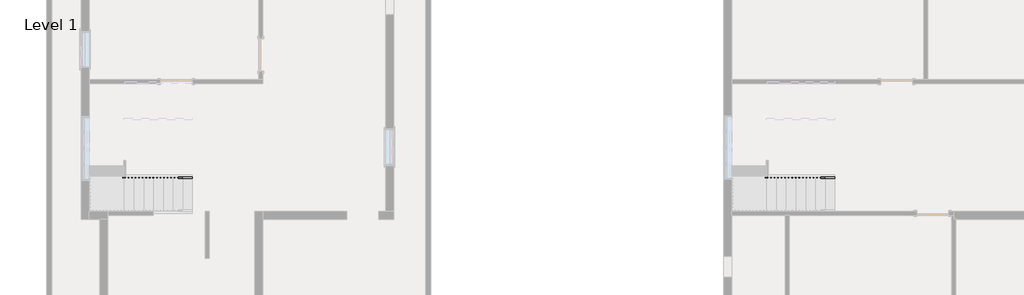
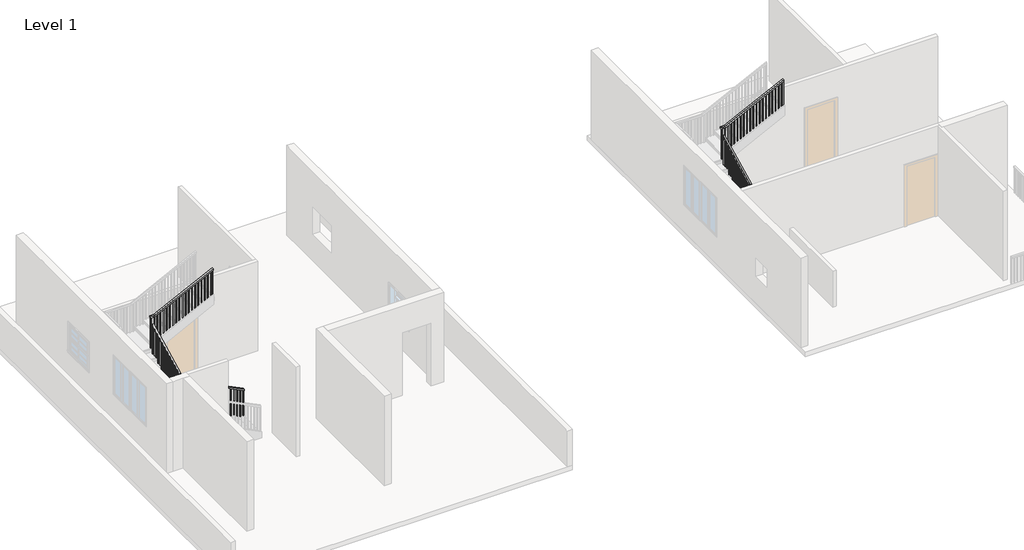
# One storey, part 4 of 8: 2 railings.
"""IFC4 building model written with IfcOpenShell, lengths in millimetres."""

from ifc_helpers import new_model, si_unit, frame, origin, place, context, project, spatial, polyline, outline, extrude, faceted_brep, element, save

model = new_model("IFC4")

# Units and contexts
model_context = context("Model", 3, world=origin())
ifc_project = project(units=[si_unit("LENGTHUNIT", "METRE", prefix="MILLI")], contexts=[model_context])

# Site, building, storey
site = spatial("IfcSite", under=ifc_project)
building = spatial("IfcBuilding", under=site)
storey = spatial("IfcBuildingStorey", under=building, Name="Level 1", Elevation=0.0)

# Railings
placement = place(None, origin())
element("IfcRailing", 1, ObjectType="Handrail - Rectangular", at=placement, inside=storey, context=model_context, shape_type="SolidModel", body=[
    faceted_brep([(-1428.1308482, -178.6399287, 1052.9454545), (-1428.1308482, -178.6399287, 996.242895), (-1428.1308482, -127.8399287, 996.242895), (-1428.1308482, -127.8399287, 1052.9454545), (-3307.7308482, -178.6399287, 1984.9785124), (-3358.5308482, -178.6399287, 1953.4660355), (-3358.5308482, -127.8399287, 1953.4660355), (-3307.7308482, -127.8399287, 1984.9785124), (-3434.7308482, -39.7364336, 2148.2942149), (-3434.7308482, -51.6399287, 2199.0942149), (-3434.7308482, 1472.3600713, 2954.7966942), (-3434.7308482, 1523.1600713, 2923.2842173), (-3383.9308482, -39.7364336, 2148.2942149), (-3383.9308482, 1523.1600713, 2923.2842173), (-3383.9308482, -51.6399287, 2199.0942149), (-3383.9308482, 1472.3600713, 2954.7966942), (-1428.1308482, 1599.3600713, 4100.9454545), (-1428.1308482, 1548.5600713, 4100.9454545), (-1428.1308482, 1548.5600713, 4044.242895), (-1428.1308482, 1599.3600713, 4044.242895), (-3295.8273531, 1599.3600713, 3118.1123967), (-3307.7308482, 1599.3600713, 3168.9123967), (-3295.8273531, 1548.5600713, 3118.1123967), (-3307.7308482, 1548.5600713, 3168.9123967), (-3307.7308482, -178.6399287, 2199.0942149), (-3358.5308482, -178.6399287, 2148.2942149), (-3358.5308482, -127.8399287, 2148.2942149), (-3307.7308482, -127.8399287, 2199.0942149), (-3434.7308482, -178.6399287, 2199.0942149), (-3434.7308482, -178.6399287, 2148.2942149), (-3383.9308482, -127.8399287, 2148.2942149), (-3383.9308482, -127.8399287, 2199.0942149), (-3434.7308482, 1472.3600713, 3168.9123967), (-3434.7308482, 1523.1600713, 3118.1123967), (-3383.9308482, 1523.1600713, 3118.1123967), (-3383.9308482, 1472.3600713, 3168.9123967), (-3434.7308482, 1599.3600713, 3168.9123967), (-3434.7308482, 1599.3600713, 3118.1123967), (-3383.9308482, 1548.5600713, 3118.1123967), (-3383.9308482, 1548.5600713, 3168.9123967)], [[[0, 1, 2, 3]], [[1, 0, 4, 5]], [[2, 1, 5, 6]], [[3, 2, 6, 7]], [[0, 3, 7, 4]], [[8, 9, 10, 11]], [[12, 8, 11, 13]], [[14, 12, 13, 15]], [[9, 14, 15, 10]], [[16, 17, 18, 19]], [[20, 21, 16, 19]], [[22, 20, 19, 18]], [[23, 22, 18, 17]], [[21, 23, 17, 16]], [[5, 4, 24, 25]], [[6, 5, 25, 26]], [[7, 6, 26, 27]], [[4, 7, 27, 24]], [[25, 24, 28, 29]], [[26, 25, 29, 30]], [[27, 26, 30, 31]], [[24, 27, 31, 28]], [[29, 28, 9, 8]], [[30, 29, 8, 12]], [[31, 30, 12, 14]], [[28, 31, 14, 9]], [[11, 10, 32, 33]], [[13, 11, 33, 34]], [[15, 13, 34, 35]], [[10, 15, 35, 32]], [[33, 32, 36, 37]], [[34, 33, 37, 38]], [[35, 34, 38, 39]], [[32, 35, 39, 36]], [[37, 36, 21, 20]], [[38, 37, 20, 22]], [[39, 38, 22, 23]], [[36, 39, 23, 21]]]),
    extrude(outline(polyline([(4023.7759528, -1469.4058482), (4014.3296718, -1488.4558482), (3048.0, -1488.4558482), (3048.0, -1469.4058482), (4023.7759528, -1469.4058482)])), frame((0.0, 1564.4350713, 0.0), z_axis=(0.0, 1.0, 0.0), x_axis=(0.0, 0.0, 1.0)), (0.0, 0.0, 1.0), 19.05),
    extrude(outline(polyline([(3973.3957875, -1571.0058482), (3963.9495065, -1590.0558482), (3048.0, -1590.0558482), (3048.0, -1571.0058482), (3973.3957875, -1571.0058482)])), frame((0.0, 1564.4350713, 0.0), z_axis=(0.0, 1.0, 0.0), x_axis=(0.0, 0.0, 1.0)), (0.0, 0.0, 1.0), 19.05),
    extrude(outline(polyline([(3923.0156222, -1672.6058482), (3913.5693412, -1691.6558482), (3048.0, -1691.6558482), (3048.0, -1672.6058482), (3923.0156222, -1672.6058482)])), frame((0.0, 1564.4350713, 0.0), z_axis=(0.0, 1.0, 0.0), x_axis=(0.0, 0.0, 1.0)), (0.0, 0.0, 1.0), 19.05),
    extrude(outline(polyline([(3872.6354569, -1774.2058482), (3863.189176, -1793.2558482), (2909.4545455, -1793.2558482), (2909.4545455, -1774.2058482), (3872.6354569, -1774.2058482)])), frame((0.0, 1564.4350713, 0.0), z_axis=(0.0, 1.0, 0.0), x_axis=(0.0, 0.0, 1.0)), (0.0, 0.0, 1.0), 19.05),
    extrude(outline(polyline([(3822.2552917, -1875.8058482), (3812.8090107, -1894.8558482), (2909.4545455, -1894.8558482), (2909.4545455, -1875.8058482), (3822.2552917, -1875.8058482)])), frame((0.0, 1564.4350713, 0.0), z_axis=(0.0, 1.0, 0.0), x_axis=(0.0, 0.0, 1.0)), (0.0, 0.0, 1.0), 19.05),
    extrude(outline(polyline([(3771.8751264, -1977.4058482), (3762.4288454, -1996.4558482), (2909.4545455, -1996.4558482), (2909.4545455, -1977.4058482), (3771.8751264, -1977.4058482)])), frame((0.0, 1564.4350713, 0.0), z_axis=(0.0, 1.0, 0.0), x_axis=(0.0, 0.0, 1.0)), (0.0, 0.0, 1.0), 19.05),
    extrude(outline(polyline([(3721.4949611, -2079.0058482), (3712.0486801, -2098.0558482), (2770.9090909, -2098.0558482), (2770.9090909, -2079.0058482), (3721.4949611, -2079.0058482)])), frame((0.0, 1564.4350713, 0.0), z_axis=(0.0, 1.0, 0.0), x_axis=(0.0, 0.0, 1.0)), (0.0, 0.0, 1.0), 19.05),
    extrude(outline(polyline([(3671.1147958, -2180.6058482), (3661.6685148, -2199.6558482), (2770.9090909, -2199.6558482), (2770.9090909, -2180.6058482), (3671.1147958, -2180.6058482)])), frame((0.0, 1564.4350713, 0.0), z_axis=(0.0, 1.0, 0.0), x_axis=(0.0, 0.0, 1.0)), (0.0, 0.0, 1.0), 19.05),
    extrude(outline(polyline([(3620.7346305, -2282.2058482), (3611.2883495, -2301.2558482), (2632.3636364, -2301.2558482), (2632.3636364, -2282.2058482), (3620.7346305, -2282.2058482)])), frame((0.0, 1564.4350713, 0.0), z_axis=(0.0, 1.0, 0.0), x_axis=(0.0, 0.0, 1.0)), (0.0, 0.0, 1.0), 19.05),
    extrude(outline(polyline([(3570.3544652, -2383.8058482), (3560.9081842, -2402.8558482), (2632.3636364, -2402.8558482), (2632.3636364, -2383.8058482), (3570.3544652, -2383.8058482)])), frame((0.0, 1564.4350713, 0.0), z_axis=(0.0, 1.0, 0.0), x_axis=(0.0, 0.0, 1.0)), (0.0, 0.0, 1.0), 19.05),
    extrude(outline(polyline([(3519.9742999, -2485.4058482), (3510.5280189, -2504.4558482), (2632.3636364, -2504.4558482), (2632.3636364, -2485.4058482), (3519.9742999, -2485.4058482)])), frame((0.0, 1564.4350713, 0.0), z_axis=(0.0, 1.0, 0.0), x_axis=(0.0, 0.0, 1.0)), (0.0, 0.0, 1.0), 19.05),
    extrude(outline(polyline([(3469.5941346, -2587.0058482), (3460.1478536, -2606.0558482), (2493.8181818, -2606.0558482), (2493.8181818, -2587.0058482), (3469.5941346, -2587.0058482)])), frame((0.0, 1564.4350713, 0.0), z_axis=(0.0, 1.0, 0.0), x_axis=(0.0, 0.0, 1.0)), (0.0, 0.0, 1.0), 19.05),
    extrude(outline(polyline([(3419.2139693, -2688.6058482), (3409.7676883, -2707.6558482), (2493.8181818, -2707.6558482), (2493.8181818, -2688.6058482), (3419.2139693, -2688.6058482)])), frame((0.0, 1564.4350713, 0.0), z_axis=(0.0, 1.0, 0.0), x_axis=(0.0, 0.0, 1.0)), (0.0, 0.0, 1.0), 19.05),
    extrude(outline(polyline([(3368.833804, -2790.2058482), (3359.3875231, -2809.2558482), (2493.8181818, -2809.2558482), (2493.8181818, -2790.2058482), (3368.833804, -2790.2058482)])), frame((0.0, 1564.4350713, 0.0), z_axis=(0.0, 1.0, 0.0), x_axis=(0.0, 0.0, 1.0)), (0.0, 0.0, 1.0), 19.05),
    extrude(outline(polyline([(3318.4536388, -2891.8058482), (3309.0073578, -2910.8558482), (2355.2727273, -2910.8558482), (2355.2727273, -2891.8058482), (3318.4536388, -2891.8058482)])), frame((0.0, 1564.4350713, 0.0), z_axis=(0.0, 1.0, 0.0), x_axis=(0.0, 0.0, 1.0)), (0.0, 0.0, 1.0), 19.05),
    extrude(outline(polyline([(3268.0734735, -2993.4058482), (3258.6271925, -3012.4558482), (2355.2727273, -3012.4558482), (2355.2727273, -2993.4058482), (3268.0734735, -2993.4058482)])), frame((0.0, 1564.4350713, 0.0), z_axis=(0.0, 1.0, 0.0), x_axis=(0.0, 0.0, 1.0)), (0.0, 0.0, 1.0), 19.05),
    extrude(outline(polyline([(3217.6933082, -3095.0058482), (3208.2470272, -3114.0558482), (2355.2727273, -3114.0558482), (2355.2727273, -3095.0058482), (3217.6933082, -3095.0058482)])), frame((0.0, 1564.4350713, 0.0), z_axis=(0.0, 1.0, 0.0), x_axis=(0.0, 0.0, 1.0)), (0.0, 0.0, 1.0), 19.05),
    extrude(outline(polyline([(3167.3131429, -3196.6058482), (3157.8668619, -3215.6558482), (2216.7272727, -3215.6558482), (2216.7272727, -3196.6058482), (3167.3131429, -3196.6058482)])), frame((0.0, 1564.4350713, 0.0), z_axis=(0.0, 1.0, 0.0), x_axis=(0.0, 0.0, 1.0)), (0.0, 0.0, 1.0), 19.05),
    extrude(outline(polyline([(3116.9329776, -3298.2058482), (3107.4866966, -3317.2558482), (2216.7272727, -3317.2558482), (2216.7272727, -3298.2058482), (3116.9329776, -3298.2058482)])), frame((0.0, 1564.4350713, 0.0), z_axis=(0.0, 1.0, 0.0), x_axis=(0.0, 0.0, 1.0)), (0.0, 0.0, 1.0), 19.05),
    extrude(outline(polyline([(1462.8350713, 2893.3709941), (1481.8850713, 2902.8172751), (1481.8850713, 1939.6363636), (1462.8350713, 1939.6363636), (1462.8350713, 2893.3709941)])), frame((-3418.8558482, 0.0, 0.0), z_axis=(1.0, 0.0, 0.0), x_axis=(0.0, 1.0, 0.0)), (0.0, 0.0, 1.0), 19.05),
    extrude(outline(polyline([(1361.2350713, 2842.9908288), (1380.2850713, 2852.4371098), (1380.2850713, 1939.6363636), (1361.2350713, 1939.6363636), (1361.2350713, 2842.9908288)])), frame((-3418.8558482, 0.0, 0.0), z_axis=(1.0, 0.0, 0.0), x_axis=(0.0, 1.0, 0.0)), (0.0, 0.0, 1.0), 19.05),
    extrude(outline(polyline([(1259.6350713, 2792.6106636), (1278.6850713, 2802.0569445), (1278.6850713, 1939.6363636), (1259.6350713, 1939.6363636), (1259.6350713, 2792.6106636)])), frame((-3418.8558482, 0.0, 0.0), z_axis=(1.0, 0.0, 0.0), x_axis=(0.0, 1.0, 0.0)), (0.0, 0.0, 1.0), 19.05),
    extrude(outline(polyline([(1158.0350713, 2742.2304983), (1177.0850713, 2751.6767793), (1177.0850713, 1801.0909091), (1158.0350713, 1801.0909091), (1158.0350713, 2742.2304983)])), frame((-3418.8558482, 0.0, 0.0), z_axis=(1.0, 0.0, 0.0), x_axis=(0.0, 1.0, 0.0)), (0.0, 0.0, 1.0), 19.05),
    extrude(outline(polyline([(1056.4350713, 2691.850333), (1075.4850713, 2701.296614), (1075.4850713, 1801.0909091), (1056.4350713, 1801.0909091), (1056.4350713, 2691.850333)])), frame((-3418.8558482, 0.0, 0.0), z_axis=(1.0, 0.0, 0.0), x_axis=(0.0, 1.0, 0.0)), (0.0, 0.0, 1.0), 19.05),
    extrude(outline(polyline([(954.8350713, 2641.4701677), (973.8850713, 2650.9164487), (973.8850713, 1662.5454545), (954.8350713, 1662.5454545), (954.8350713, 2641.4701677)])), frame((-3418.8558482, 0.0, 0.0), z_axis=(1.0, 0.0, 0.0), x_axis=(0.0, 1.0, 0.0)), (0.0, 0.0, 1.0), 19.05),
    extrude(outline(polyline([(853.2350713, 2591.0900024), (872.2850713, 2600.5362834), (872.2850713, 1662.5454545), (853.2350713, 1662.5454545), (853.2350713, 2591.0900024)])), frame((-3418.8558482, 0.0, 0.0), z_axis=(1.0, 0.0, 0.0), x_axis=(0.0, 1.0, 0.0)), (0.0, 0.0, 1.0), 19.05),
    extrude(outline(polyline([(751.6350713, 2540.7098371), (770.6850713, 2550.1561181), (770.6850713, 1662.5454545), (751.6350713, 1662.5454545), (751.6350713, 2540.7098371)])), frame((-3418.8558482, 0.0, 0.0), z_axis=(1.0, 0.0, 0.0), x_axis=(0.0, 1.0, 0.0)), (0.0, 0.0, 1.0), 19.05),
    extrude(outline(polyline([(650.0350713, 2490.3296718), (669.0850713, 2499.7759528), (669.0850713, 1524.0), (650.0350713, 1524.0), (650.0350713, 2490.3296718)])), frame((-3418.8558482, 0.0, 0.0), z_axis=(1.0, 0.0, 0.0), x_axis=(0.0, 1.0, 0.0)), (0.0, 0.0, 1.0), 19.05),
    extrude(outline(polyline([(548.4350713, 2439.9495065), (567.4850713, 2449.3957875), (567.4850713, 1524.0), (548.4350713, 1524.0), (548.4350713, 2439.9495065)])), frame((-3418.8558482, 0.0, 0.0), z_axis=(1.0, 0.0, 0.0), x_axis=(0.0, 1.0, 0.0)), (0.0, 0.0, 1.0), 19.05),
    extrude(outline(polyline([(446.8350713, 2389.5693412), (465.8850713, 2399.0156222), (465.8850713, 1524.0), (446.8350713, 1524.0), (446.8350713, 2389.5693412)])), frame((-3418.8558482, 0.0, 0.0), z_axis=(1.0, 0.0, 0.0), x_axis=(0.0, 1.0, 0.0)), (0.0, 0.0, 1.0), 19.05),
    extrude(outline(polyline([(345.2350713, 2339.189176), (364.2850713, 2348.6354569), (364.2850713, 1385.4545455), (345.2350713, 1385.4545455), (345.2350713, 2339.189176)])), frame((-3418.8558482, 0.0, 0.0), z_axis=(1.0, 0.0, 0.0), x_axis=(0.0, 1.0, 0.0)), (0.0, 0.0, 1.0), 19.05),
    extrude(outline(polyline([(243.6350713, 2288.8090107), (262.6850713, 2298.2552917), (262.6850713, 1385.4545455), (243.6350713, 1385.4545455), (243.6350713, 2288.8090107)])), frame((-3418.8558482, 0.0, 0.0), z_axis=(1.0, 0.0, 0.0), x_axis=(0.0, 1.0, 0.0)), (0.0, 0.0, 1.0), 19.05),
    extrude(outline(polyline([(142.0350713, 2238.4288454), (161.0850713, 2247.8751264), (161.0850713, 1385.4545455), (142.0350713, 1385.4545455), (142.0350713, 2238.4288454)])), frame((-3418.8558482, 0.0, 0.0), z_axis=(1.0, 0.0, 0.0), x_axis=(0.0, 1.0, 0.0)), (0.0, 0.0, 1.0), 19.05),
    extrude(outline(polyline([(40.4350713, 2188.0486801), (59.4850713, 2197.4949611), (59.4850713, 1246.9090909), (40.4350713, 1246.9090909), (40.4350713, 2188.0486801)])), frame((-3418.8558482, 0.0, 0.0), z_axis=(1.0, 0.0, 0.0), x_axis=(0.0, 1.0, 0.0)), (0.0, 0.0, 1.0), 19.05),
    extrude(outline(polyline([(-61.1649287, 2137.6685148), (-42.1149287, 2147.1147958), (-42.1149287, 1246.9090909), (-61.1649287, 1246.9090909), (-61.1649287, 2137.6685148)])), frame((-3418.8558482, 0.0, 0.0), z_axis=(1.0, 0.0, 0.0), x_axis=(0.0, 1.0, 0.0)), (0.0, 0.0, 1.0), 19.05),
    extrude(outline(polyline([(-3349.0058482, -143.7149287), (-3349.0058482, -162.7649287), (-3368.0558482, -162.7649287), (-3368.0558482, -143.7149287), (-3349.0058482, -143.7149287)])), frame((0.0, 0.0, 969.8181818), z_axis=(0.0, 0.0, 1.0), x_axis=(1.0, 0.0, 0.0)), (0.0, 0.0, 1.0), 1178.4760331),
    extrude(outline(polyline([(1898.3627297, -3247.4058482), (1907.8090107, -3266.4558482), (969.8181818, -3266.4558482), (969.8181818, -3247.4058482), (1898.3627297, -3247.4058482)])), frame((0.0, -162.7649287, 0.0), z_axis=(0.0, 1.0, 0.0), x_axis=(0.0, 0.0, 1.0)), (0.0, 0.0, 1.0), 19.05),
    extrude(outline(polyline([(1847.9825644, -3145.8058482), (1857.4288454, -3164.8558482), (969.8181818, -3164.8558482), (969.8181818, -3145.8058482), (1847.9825644, -3145.8058482)])), frame((0.0, -162.7649287, 0.0), z_axis=(0.0, 1.0, 0.0), x_axis=(0.0, 0.0, 1.0)), (0.0, 0.0, 1.0), 19.05),
    extrude(outline(polyline([(1797.6023991, -3044.2058482), (1807.0486801, -3063.2558482), (831.2727273, -3063.2558482), (831.2727273, -3044.2058482), (1797.6023991, -3044.2058482)])), frame((0.0, -162.7649287, 0.0), z_axis=(0.0, 1.0, 0.0), x_axis=(0.0, 0.0, 1.0)), (0.0, 0.0, 1.0), 19.05),
    extrude(outline(polyline([(1747.2222338, -2942.6058482), (1756.6685148, -2961.6558482), (831.2727273, -2961.6558482), (831.2727273, -2942.6058482), (1747.2222338, -2942.6058482)])), frame((0.0, -162.7649287, 0.0), z_axis=(0.0, 1.0, 0.0), x_axis=(0.0, 0.0, 1.0)), (0.0, 0.0, 1.0), 19.05),
    extrude(outline(polyline([(1696.8420685, -2841.0058482), (1706.2883495, -2860.0558482), (831.2727273, -2860.0558482), (831.2727273, -2841.0058482), (1696.8420685, -2841.0058482)])), frame((0.0, -162.7649287, 0.0), z_axis=(0.0, 1.0, 0.0), x_axis=(0.0, 0.0, 1.0)), (0.0, 0.0, 1.0), 19.05),
    extrude(outline(polyline([(1646.4619032, -2739.4058482), (1655.9081842, -2758.4558482), (692.7272727, -2758.4558482), (692.7272727, -2739.4058482), (1646.4619032, -2739.4058482)])), frame((0.0, -162.7649287, 0.0), z_axis=(0.0, 1.0, 0.0), x_axis=(0.0, 0.0, 1.0)), (0.0, 0.0, 1.0), 19.05),
    extrude(outline(polyline([(1596.0817379, -2637.8058482), (1605.5280189, -2656.8558482), (692.7272727, -2656.8558482), (692.7272727, -2637.8058482), (1596.0817379, -2637.8058482)])), frame((0.0, -162.7649287, 0.0), z_axis=(0.0, 1.0, 0.0), x_axis=(0.0, 0.0, 1.0)), (0.0, 0.0, 1.0), 19.05),
    extrude(outline(polyline([(1545.7015726, -2536.2058482), (1555.1478536, -2555.2558482), (692.7272727, -2555.2558482), (692.7272727, -2536.2058482), (1545.7015726, -2536.2058482)])), frame((0.0, -162.7649287, 0.0), z_axis=(0.0, 1.0, 0.0), x_axis=(0.0, 0.0, 1.0)), (0.0, 0.0, 1.0), 19.05),
    extrude(outline(polyline([(1495.3214074, -2434.6058482), (1504.7676883, -2453.6558482), (554.1818182, -2453.6558482), (554.1818182, -2434.6058482), (1495.3214074, -2434.6058482)])), frame((0.0, -162.7649287, 0.0), z_axis=(0.0, 1.0, 0.0), x_axis=(0.0, 0.0, 1.0)), (0.0, 0.0, 1.0), 19.05),
    extrude(outline(polyline([(1444.9412421, -2333.0058482), (1454.3875231, -2352.0558482), (554.1818182, -2352.0558482), (554.1818182, -2333.0058482), (1444.9412421, -2333.0058482)])), frame((0.0, -162.7649287, 0.0), z_axis=(0.0, 1.0, 0.0), x_axis=(0.0, 0.0, 1.0)), (0.0, 0.0, 1.0), 19.05),
    extrude(outline(polyline([(1394.5610768, -2231.4058482), (1404.0073578, -2250.4558482), (415.6363636, -2250.4558482), (415.6363636, -2231.4058482), (1394.5610768, -2231.4058482)])), frame((0.0, -162.7649287, 0.0), z_axis=(0.0, 1.0, 0.0), x_axis=(0.0, 0.0, 1.0)), (0.0, 0.0, 1.0), 19.05),
    extrude(outline(polyline([(1344.1809115, -2129.8058482), (1353.6271925, -2148.8558482), (415.6363636, -2148.8558482), (415.6363636, -2129.8058482), (1344.1809115, -2129.8058482)])), frame((0.0, -162.7649287, 0.0), z_axis=(0.0, 1.0, 0.0), x_axis=(0.0, 0.0, 1.0)), (0.0, 0.0, 1.0), 19.05),
    extrude(outline(polyline([(1293.8007462, -2028.2058482), (1303.2470272, -2047.2558482), (415.6363636, -2047.2558482), (415.6363636, -2028.2058482), (1293.8007462, -2028.2058482)])), frame((0.0, -162.7649287, 0.0), z_axis=(0.0, 1.0, 0.0), x_axis=(0.0, 0.0, 1.0)), (0.0, 0.0, 1.0), 19.05),
    extrude(outline(polyline([(1243.4205809, -1926.6058482), (1252.8668619, -1945.6558482), (277.0909091, -1945.6558482), (277.0909091, -1926.6058482), (1243.4205809, -1926.6058482)])), frame((0.0, -162.7649287, 0.0), z_axis=(0.0, 1.0, 0.0), x_axis=(0.0, 0.0, 1.0)), (0.0, 0.0, 1.0), 19.05),
    extrude(outline(polyline([(1193.0404156, -1825.0058482), (1202.4866966, -1844.0558482), (277.0909091, -1844.0558482), (277.0909091, -1825.0058482), (1193.0404156, -1825.0058482)])), frame((0.0, -162.7649287, 0.0), z_axis=(0.0, 1.0, 0.0), x_axis=(0.0, 0.0, 1.0)), (0.0, 0.0, 1.0), 19.05),
    extrude(outline(polyline([(1142.6602503, -1723.4058482), (1152.1065313, -1742.4558482), (277.0909091, -1742.4558482), (277.0909091, -1723.4058482), (1142.6602503, -1723.4058482)])), frame((0.0, -162.7649287, 0.0), z_axis=(0.0, 1.0, 0.0), x_axis=(0.0, 0.0, 1.0)), (0.0, 0.0, 1.0), 19.05),
    extrude(outline(polyline([(1092.280085, -1621.8058482), (1101.726366, -1640.8558482), (138.5454545, -1640.8558482), (138.5454545, -1621.8058482), (1092.280085, -1621.8058482)])), frame((0.0, -162.7649287, 0.0), z_axis=(0.0, 1.0, 0.0), x_axis=(0.0, 0.0, 1.0)), (0.0, 0.0, 1.0), 19.05),
    extrude(outline(polyline([(1041.8999198, -1520.2058482), (1051.3462007, -1539.2558482), (138.5454545, -1539.2558482), (138.5454545, -1520.2058482), (1041.8999198, -1520.2058482)])), frame((0.0, -162.7649287, 0.0), z_axis=(0.0, 1.0, 0.0), x_axis=(0.0, 0.0, 1.0)), (0.0, 0.0, 1.0), 19.05),
    extrude(outline(polyline([(-3399.8058482, 1564.4350713), (-3418.8558482, 1564.4350713), (-3418.8558482, 1583.4850713), (-3399.8058482, 1583.4850713), (-3399.8058482, 1564.4350713)])), frame((0.0, 0.0, 2078.1818182), z_axis=(0.0, 0.0, 1.0), x_axis=(1.0, 0.0, 0.0)), (0.0, 0.0, 1.0), 1039.9305785),
    extrude(outline(polyline([(-3399.8058482, -143.7149287), (-3399.8058482, -162.7649287), (-3418.8558482, -162.7649287), (-3418.8558482, -143.7149287), (-3399.8058482, -143.7149287)])), frame((0.0, 0.0, 1108.3636364), z_axis=(0.0, 0.0, 1.0), x_axis=(1.0, 0.0, 0.0)), (0.0, 0.0, 1.0), 1039.9305785),
    extrude(outline(polyline([(4044.242895, -1428.1308482), (4034.796614, -1447.1808482), (3048.0, -1447.1808482), (3048.0, -1428.1308482), (4044.242895, -1428.1308482)])), frame((0.0, 1564.4350713, 0.0), z_axis=(0.0, 1.0, 0.0), x_axis=(0.0, 0.0, 1.0)), (0.0, 0.0, 1.0), 19.05),
    extrude(outline(polyline([(996.242895, -1428.1308482), (1005.689176, -1447.1808482), (138.5454545, -1447.1808482), (138.5454545, -1428.1308482), (996.242895, -1428.1308482)])), frame((0.0, -162.7649287, 0.0), z_axis=(0.0, 1.0, 0.0), x_axis=(0.0, 0.0, 1.0)), (0.0, 0.0, 1.0), 19.05),
])
element("IfcRailing", 2, ObjectType="Handrail - Rectangular", at=placement, inside=storey, context=model_context, shape_type="SolidModel", body=[
    faceted_brep([(-19769.8789184, -178.6399287, 1052.9454545), (-19769.8789184, -178.6399287, 996.242895), (-19769.8789184, -127.8399287, 996.242895), (-19769.8789184, -127.8399287, 1052.9454545), (-21649.4789184, -178.6399287, 1984.9785124), (-21700.2789184, -178.6399287, 1953.4660355), (-21700.2789184, -127.8399287, 1953.4660355), (-21649.4789184, -127.8399287, 1984.9785124), (-21776.4789184, -39.7364336, 2148.2942149), (-21776.4789184, -51.6399287, 2199.0942149), (-21776.4789184, 1472.3600713, 2954.7966942), (-21776.4789184, 1523.1600713, 2923.2842173), (-21725.6789184, -39.7364336, 2148.2942149), (-21725.6789184, 1523.1600713, 2923.2842173), (-21725.6789184, -51.6399287, 2199.0942149), (-21725.6789184, 1472.3600713, 2954.7966942), (-19769.8789184, 1599.3600713, 4100.9454545), (-19769.8789184, 1548.5600713, 4100.9454545), (-19769.8789184, 1548.5600713, 4044.242895), (-19769.8789184, 1599.3600713, 4044.242895), (-21637.5754233, 1599.3600713, 3118.1123967), (-21649.4789184, 1599.3600713, 3168.9123967), (-21637.5754233, 1548.5600713, 3118.1123967), (-21649.4789184, 1548.5600713, 3168.9123967), (-21649.4789184, -178.6399287, 2199.0942149), (-21700.2789184, -178.6399287, 2148.2942149), (-21700.2789184, -127.8399287, 2148.2942149), (-21649.4789184, -127.8399287, 2199.0942149), (-21776.4789184, -178.6399287, 2199.0942149), (-21776.4789184, -178.6399287, 2148.2942149), (-21725.6789184, -127.8399287, 2148.2942149), (-21725.6789184, -127.8399287, 2199.0942149), (-21776.4789184, 1472.3600713, 3168.9123967), (-21776.4789184, 1523.1600713, 3118.1123967), (-21725.6789184, 1523.1600713, 3118.1123967), (-21725.6789184, 1472.3600713, 3168.9123967), (-21776.4789184, 1599.3600713, 3168.9123967), (-21776.4789184, 1599.3600713, 3118.1123967), (-21725.6789184, 1548.5600713, 3118.1123967), (-21725.6789184, 1548.5600713, 3168.9123967)], [[[0, 1, 2, 3]], [[1, 0, 4, 5]], [[2, 1, 5, 6]], [[3, 2, 6, 7]], [[0, 3, 7, 4]], [[8, 9, 10, 11]], [[12, 8, 11, 13]], [[14, 12, 13, 15]], [[9, 14, 15, 10]], [[16, 17, 18, 19]], [[20, 21, 16, 19]], [[22, 20, 19, 18]], [[23, 22, 18, 17]], [[21, 23, 17, 16]], [[5, 4, 24, 25]], [[6, 5, 25, 26]], [[7, 6, 26, 27]], [[4, 7, 27, 24]], [[25, 24, 28, 29]], [[26, 25, 29, 30]], [[27, 26, 30, 31]], [[24, 27, 31, 28]], [[29, 28, 9, 8]], [[30, 29, 8, 12]], [[31, 30, 12, 14]], [[28, 31, 14, 9]], [[11, 10, 32, 33]], [[13, 11, 33, 34]], [[15, 13, 34, 35]], [[10, 15, 35, 32]], [[33, 32, 36, 37]], [[34, 33, 37, 38]], [[35, 34, 38, 39]], [[32, 35, 39, 36]], [[37, 36, 21, 20]], [[38, 37, 20, 22]], [[39, 38, 22, 23]], [[36, 39, 23, 21]]]),
    extrude(outline(polyline([(4023.7759528, -19811.1539184), (4014.3296718, -19830.2039184), (3048.0, -19830.2039184), (3048.0, -19811.1539184), (4023.7759528, -19811.1539184)])), frame((0.0, 1564.4350713, 0.0), z_axis=(0.0, 1.0, 0.0), x_axis=(0.0, 0.0, 1.0)), (0.0, 0.0, 1.0), 19.05),
    extrude(outline(polyline([(3973.3957875, -19912.7539184), (3963.9495065, -19931.8039184), (3048.0, -19931.8039184), (3048.0, -19912.7539184), (3973.3957875, -19912.7539184)])), frame((0.0, 1564.4350713, 0.0), z_axis=(0.0, 1.0, 0.0), x_axis=(0.0, 0.0, 1.0)), (0.0, 0.0, 1.0), 19.05),
    extrude(outline(polyline([(3923.0156222, -20014.3539184), (3913.5693412, -20033.4039184), (3048.0, -20033.4039184), (3048.0, -20014.3539184), (3923.0156222, -20014.3539184)])), frame((0.0, 1564.4350713, 0.0), z_axis=(0.0, 1.0, 0.0), x_axis=(0.0, 0.0, 1.0)), (0.0, 0.0, 1.0), 19.05),
    extrude(outline(polyline([(3872.6354569, -20115.9539184), (3863.189176, -20135.0039184), (2909.4545455, -20135.0039184), (2909.4545455, -20115.9539184), (3872.6354569, -20115.9539184)])), frame((0.0, 1564.4350713, 0.0), z_axis=(0.0, 1.0, 0.0), x_axis=(0.0, 0.0, 1.0)), (0.0, 0.0, 1.0), 19.05),
    extrude(outline(polyline([(3822.2552917, -20217.5539184), (3812.8090107, -20236.6039184), (2909.4545455, -20236.6039184), (2909.4545455, -20217.5539184), (3822.2552917, -20217.5539184)])), frame((0.0, 1564.4350713, 0.0), z_axis=(0.0, 1.0, 0.0), x_axis=(0.0, 0.0, 1.0)), (0.0, 0.0, 1.0), 19.05),
    extrude(outline(polyline([(3771.8751264, -20319.1539184), (3762.4288454, -20338.2039184), (2909.4545455, -20338.2039184), (2909.4545455, -20319.1539184), (3771.8751264, -20319.1539184)])), frame((0.0, 1564.4350713, 0.0), z_axis=(0.0, 1.0, 0.0), x_axis=(0.0, 0.0, 1.0)), (0.0, 0.0, 1.0), 19.05),
    extrude(outline(polyline([(3721.4949611, -20420.7539184), (3712.0486801, -20439.8039184), (2770.9090909, -20439.8039184), (2770.9090909, -20420.7539184), (3721.4949611, -20420.7539184)])), frame((0.0, 1564.4350713, 0.0), z_axis=(0.0, 1.0, 0.0), x_axis=(0.0, 0.0, 1.0)), (0.0, 0.0, 1.0), 19.05),
    extrude(outline(polyline([(3671.1147958, -20522.3539184), (3661.6685148, -20541.4039184), (2770.9090909, -20541.4039184), (2770.9090909, -20522.3539184), (3671.1147958, -20522.3539184)])), frame((0.0, 1564.4350713, 0.0), z_axis=(0.0, 1.0, 0.0), x_axis=(0.0, 0.0, 1.0)), (0.0, 0.0, 1.0), 19.05),
    extrude(outline(polyline([(3620.7346305, -20623.9539184), (3611.2883495, -20643.0039184), (2632.3636364, -20643.0039184), (2632.3636364, -20623.9539184), (3620.7346305, -20623.9539184)])), frame((0.0, 1564.4350713, 0.0), z_axis=(0.0, 1.0, 0.0), x_axis=(0.0, 0.0, 1.0)), (0.0, 0.0, 1.0), 19.05),
    extrude(outline(polyline([(3570.3544652, -20725.5539184), (3560.9081842, -20744.6039184), (2632.3636364, -20744.6039184), (2632.3636364, -20725.5539184), (3570.3544652, -20725.5539184)])), frame((0.0, 1564.4350713, 0.0), z_axis=(0.0, 1.0, 0.0), x_axis=(0.0, 0.0, 1.0)), (0.0, 0.0, 1.0), 19.05),
    extrude(outline(polyline([(3519.9742999, -20827.1539184), (3510.5280189, -20846.2039184), (2632.3636364, -20846.2039184), (2632.3636364, -20827.1539184), (3519.9742999, -20827.1539184)])), frame((0.0, 1564.4350713, 0.0), z_axis=(0.0, 1.0, 0.0), x_axis=(0.0, 0.0, 1.0)), (0.0, 0.0, 1.0), 19.05),
    extrude(outline(polyline([(3469.5941346, -20928.7539184), (3460.1478536, -20947.8039184), (2493.8181818, -20947.8039184), (2493.8181818, -20928.7539184), (3469.5941346, -20928.7539184)])), frame((0.0, 1564.4350713, 0.0), z_axis=(0.0, 1.0, 0.0), x_axis=(0.0, 0.0, 1.0)), (0.0, 0.0, 1.0), 19.05),
    extrude(outline(polyline([(3419.2139693, -21030.3539184), (3409.7676883, -21049.4039184), (2493.8181818, -21049.4039184), (2493.8181818, -21030.3539184), (3419.2139693, -21030.3539184)])), frame((0.0, 1564.4350713, 0.0), z_axis=(0.0, 1.0, 0.0), x_axis=(0.0, 0.0, 1.0)), (0.0, 0.0, 1.0), 19.05),
    extrude(outline(polyline([(3368.833804, -21131.9539184), (3359.3875231, -21151.0039184), (2493.8181818, -21151.0039184), (2493.8181818, -21131.9539184), (3368.833804, -21131.9539184)])), frame((0.0, 1564.4350713, 0.0), z_axis=(0.0, 1.0, 0.0), x_axis=(0.0, 0.0, 1.0)), (0.0, 0.0, 1.0), 19.05),
    extrude(outline(polyline([(3318.4536388, -21233.5539184), (3309.0073578, -21252.6039184), (2355.2727273, -21252.6039184), (2355.2727273, -21233.5539184), (3318.4536388, -21233.5539184)])), frame((0.0, 1564.4350713, 0.0), z_axis=(0.0, 1.0, 0.0), x_axis=(0.0, 0.0, 1.0)), (0.0, 0.0, 1.0), 19.05),
    extrude(outline(polyline([(3268.0734735, -21335.1539184), (3258.6271925, -21354.2039184), (2355.2727273, -21354.2039184), (2355.2727273, -21335.1539184), (3268.0734735, -21335.1539184)])), frame((0.0, 1564.4350713, 0.0), z_axis=(0.0, 1.0, 0.0), x_axis=(0.0, 0.0, 1.0)), (0.0, 0.0, 1.0), 19.05),
    extrude(outline(polyline([(3217.6933082, -21436.7539184), (3208.2470272, -21455.8039184), (2355.2727273, -21455.8039184), (2355.2727273, -21436.7539184), (3217.6933082, -21436.7539184)])), frame((0.0, 1564.4350713, 0.0), z_axis=(0.0, 1.0, 0.0), x_axis=(0.0, 0.0, 1.0)), (0.0, 0.0, 1.0), 19.05),
    extrude(outline(polyline([(3167.3131429, -21538.3539184), (3157.8668619, -21557.4039184), (2216.7272727, -21557.4039184), (2216.7272727, -21538.3539184), (3167.3131429, -21538.3539184)])), frame((0.0, 1564.4350713, 0.0), z_axis=(0.0, 1.0, 0.0), x_axis=(0.0, 0.0, 1.0)), (0.0, 0.0, 1.0), 19.05),
    extrude(outline(polyline([(3116.9329776, -21639.9539184), (3107.4866966, -21659.0039184), (2216.7272727, -21659.0039184), (2216.7272727, -21639.9539184), (3116.9329776, -21639.9539184)])), frame((0.0, 1564.4350713, 0.0), z_axis=(0.0, 1.0, 0.0), x_axis=(0.0, 0.0, 1.0)), (0.0, 0.0, 1.0), 19.05),
    extrude(outline(polyline([(1462.8350713, 2893.3709941), (1481.8850713, 2902.8172751), (1481.8850713, 1939.6363636), (1462.8350713, 1939.6363636), (1462.8350713, 2893.3709941)])), frame((-21760.6039184, 0.0, 0.0), z_axis=(1.0, 0.0, 0.0), x_axis=(0.0, 1.0, 0.0)), (0.0, 0.0, 1.0), 19.05),
    extrude(outline(polyline([(1361.2350713, 2842.9908288), (1380.2850713, 2852.4371098), (1380.2850713, 1939.6363636), (1361.2350713, 1939.6363636), (1361.2350713, 2842.9908288)])), frame((-21760.6039184, 0.0, 0.0), z_axis=(1.0, 0.0, 0.0), x_axis=(0.0, 1.0, 0.0)), (0.0, 0.0, 1.0), 19.05),
    extrude(outline(polyline([(1259.6350713, 2792.6106636), (1278.6850713, 2802.0569445), (1278.6850713, 1939.6363636), (1259.6350713, 1939.6363636), (1259.6350713, 2792.6106636)])), frame((-21760.6039184, 0.0, 0.0), z_axis=(1.0, 0.0, 0.0), x_axis=(0.0, 1.0, 0.0)), (0.0, 0.0, 1.0), 19.05),
    extrude(outline(polyline([(1158.0350713, 2742.2304983), (1177.0850713, 2751.6767793), (1177.0850713, 1801.0909091), (1158.0350713, 1801.0909091), (1158.0350713, 2742.2304983)])), frame((-21760.6039184, 0.0, 0.0), z_axis=(1.0, 0.0, 0.0), x_axis=(0.0, 1.0, 0.0)), (0.0, 0.0, 1.0), 19.05),
    extrude(outline(polyline([(1056.4350713, 2691.850333), (1075.4850713, 2701.296614), (1075.4850713, 1801.0909091), (1056.4350713, 1801.0909091), (1056.4350713, 2691.850333)])), frame((-21760.6039184, 0.0, 0.0), z_axis=(1.0, 0.0, 0.0), x_axis=(0.0, 1.0, 0.0)), (0.0, 0.0, 1.0), 19.05),
    extrude(outline(polyline([(954.8350713, 2641.4701677), (973.8850713, 2650.9164487), (973.8850713, 1662.5454545), (954.8350713, 1662.5454545), (954.8350713, 2641.4701677)])), frame((-21760.6039184, 0.0, 0.0), z_axis=(1.0, 0.0, 0.0), x_axis=(0.0, 1.0, 0.0)), (0.0, 0.0, 1.0), 19.05),
    extrude(outline(polyline([(853.2350713, 2591.0900024), (872.2850713, 2600.5362834), (872.2850713, 1662.5454545), (853.2350713, 1662.5454545), (853.2350713, 2591.0900024)])), frame((-21760.6039184, 0.0, 0.0), z_axis=(1.0, 0.0, 0.0), x_axis=(0.0, 1.0, 0.0)), (0.0, 0.0, 1.0), 19.05),
    extrude(outline(polyline([(751.6350713, 2540.7098371), (770.6850713, 2550.1561181), (770.6850713, 1662.5454545), (751.6350713, 1662.5454545), (751.6350713, 2540.7098371)])), frame((-21760.6039184, 0.0, 0.0), z_axis=(1.0, 0.0, 0.0), x_axis=(0.0, 1.0, 0.0)), (0.0, 0.0, 1.0), 19.05),
    extrude(outline(polyline([(650.0350713, 2490.3296718), (669.0850713, 2499.7759528), (669.0850713, 1524.0), (650.0350713, 1524.0), (650.0350713, 2490.3296718)])), frame((-21760.6039184, 0.0, 0.0), z_axis=(1.0, 0.0, 0.0), x_axis=(0.0, 1.0, 0.0)), (0.0, 0.0, 1.0), 19.05),
    extrude(outline(polyline([(548.4350713, 2439.9495065), (567.4850713, 2449.3957875), (567.4850713, 1524.0), (548.4350713, 1524.0), (548.4350713, 2439.9495065)])), frame((-21760.6039184, 0.0, 0.0), z_axis=(1.0, 0.0, 0.0), x_axis=(0.0, 1.0, 0.0)), (0.0, 0.0, 1.0), 19.05),
    extrude(outline(polyline([(446.8350713, 2389.5693412), (465.8850713, 2399.0156222), (465.8850713, 1524.0), (446.8350713, 1524.0), (446.8350713, 2389.5693412)])), frame((-21760.6039184, 0.0, 0.0), z_axis=(1.0, 0.0, 0.0), x_axis=(0.0, 1.0, 0.0)), (0.0, 0.0, 1.0), 19.05),
    extrude(outline(polyline([(345.2350713, 2339.189176), (364.2850713, 2348.6354569), (364.2850713, 1385.4545455), (345.2350713, 1385.4545455), (345.2350713, 2339.189176)])), frame((-21760.6039184, 0.0, 0.0), z_axis=(1.0, 0.0, 0.0), x_axis=(0.0, 1.0, 0.0)), (0.0, 0.0, 1.0), 19.05),
    extrude(outline(polyline([(243.6350713, 2288.8090107), (262.6850713, 2298.2552917), (262.6850713, 1385.4545455), (243.6350713, 1385.4545455), (243.6350713, 2288.8090107)])), frame((-21760.6039184, 0.0, 0.0), z_axis=(1.0, 0.0, 0.0), x_axis=(0.0, 1.0, 0.0)), (0.0, 0.0, 1.0), 19.05),
    extrude(outline(polyline([(142.0350713, 2238.4288454), (161.0850713, 2247.8751264), (161.0850713, 1385.4545455), (142.0350713, 1385.4545455), (142.0350713, 2238.4288454)])), frame((-21760.6039184, 0.0, 0.0), z_axis=(1.0, 0.0, 0.0), x_axis=(0.0, 1.0, 0.0)), (0.0, 0.0, 1.0), 19.05),
    extrude(outline(polyline([(40.4350713, 2188.0486801), (59.4850713, 2197.4949611), (59.4850713, 1246.9090909), (40.4350713, 1246.9090909), (40.4350713, 2188.0486801)])), frame((-21760.6039184, 0.0, 0.0), z_axis=(1.0, 0.0, 0.0), x_axis=(0.0, 1.0, 0.0)), (0.0, 0.0, 1.0), 19.05),
    extrude(outline(polyline([(-61.1649287, 2137.6685148), (-42.1149287, 2147.1147958), (-42.1149287, 1246.9090909), (-61.1649287, 1246.9090909), (-61.1649287, 2137.6685148)])), frame((-21760.6039184, 0.0, 0.0), z_axis=(1.0, 0.0, 0.0), x_axis=(0.0, 1.0, 0.0)), (0.0, 0.0, 1.0), 19.05),
    extrude(outline(polyline([(-21690.7539184, -143.7149287), (-21690.7539184, -162.7649287), (-21709.8039184, -162.7649287), (-21709.8039184, -143.7149287), (-21690.7539184, -143.7149287)])), frame((0.0, 0.0, 969.8181818), z_axis=(0.0, 0.0, 1.0), x_axis=(1.0, 0.0, 0.0)), (0.0, 0.0, 1.0), 1178.4760331),
    extrude(outline(polyline([(1898.3627297, -21589.1539184), (1907.8090107, -21608.2039184), (969.8181818, -21608.2039184), (969.8181818, -21589.1539184), (1898.3627297, -21589.1539184)])), frame((0.0, -162.7649287, 0.0), z_axis=(0.0, 1.0, 0.0), x_axis=(0.0, 0.0, 1.0)), (0.0, 0.0, 1.0), 19.05),
    extrude(outline(polyline([(1847.9825644, -21487.5539184), (1857.4288454, -21506.6039184), (969.8181818, -21506.6039184), (969.8181818, -21487.5539184), (1847.9825644, -21487.5539184)])), frame((0.0, -162.7649287, 0.0), z_axis=(0.0, 1.0, 0.0), x_axis=(0.0, 0.0, 1.0)), (0.0, 0.0, 1.0), 19.05),
    extrude(outline(polyline([(1797.6023991, -21385.9539184), (1807.0486801, -21405.0039184), (831.2727273, -21405.0039184), (831.2727273, -21385.9539184), (1797.6023991, -21385.9539184)])), frame((0.0, -162.7649287, 0.0), z_axis=(0.0, 1.0, 0.0), x_axis=(0.0, 0.0, 1.0)), (0.0, 0.0, 1.0), 19.05),
    extrude(outline(polyline([(1747.2222338, -21284.3539184), (1756.6685148, -21303.4039184), (831.2727273, -21303.4039184), (831.2727273, -21284.3539184), (1747.2222338, -21284.3539184)])), frame((0.0, -162.7649287, 0.0), z_axis=(0.0, 1.0, 0.0), x_axis=(0.0, 0.0, 1.0)), (0.0, 0.0, 1.0), 19.05),
    extrude(outline(polyline([(1696.8420685, -21182.7539184), (1706.2883495, -21201.8039184), (831.2727273, -21201.8039184), (831.2727273, -21182.7539184), (1696.8420685, -21182.7539184)])), frame((0.0, -162.7649287, 0.0), z_axis=(0.0, 1.0, 0.0), x_axis=(0.0, 0.0, 1.0)), (0.0, 0.0, 1.0), 19.05),
    extrude(outline(polyline([(1646.4619032, -21081.1539184), (1655.9081842, -21100.2039184), (692.7272727, -21100.2039184), (692.7272727, -21081.1539184), (1646.4619032, -21081.1539184)])), frame((0.0, -162.7649287, 0.0), z_axis=(0.0, 1.0, 0.0), x_axis=(0.0, 0.0, 1.0)), (0.0, 0.0, 1.0), 19.05),
    extrude(outline(polyline([(1596.0817379, -20979.5539184), (1605.5280189, -20998.6039184), (692.7272727, -20998.6039184), (692.7272727, -20979.5539184), (1596.0817379, -20979.5539184)])), frame((0.0, -162.7649287, 0.0), z_axis=(0.0, 1.0, 0.0), x_axis=(0.0, 0.0, 1.0)), (0.0, 0.0, 1.0), 19.05),
    extrude(outline(polyline([(1545.7015726, -20877.9539184), (1555.1478536, -20897.0039184), (692.7272727, -20897.0039184), (692.7272727, -20877.9539184), (1545.7015726, -20877.9539184)])), frame((0.0, -162.7649287, 0.0), z_axis=(0.0, 1.0, 0.0), x_axis=(0.0, 0.0, 1.0)), (0.0, 0.0, 1.0), 19.05),
    extrude(outline(polyline([(1495.3214074, -20776.3539184), (1504.7676883, -20795.4039184), (554.1818182, -20795.4039184), (554.1818182, -20776.3539184), (1495.3214074, -20776.3539184)])), frame((0.0, -162.7649287, 0.0), z_axis=(0.0, 1.0, 0.0), x_axis=(0.0, 0.0, 1.0)), (0.0, 0.0, 1.0), 19.05),
    extrude(outline(polyline([(1444.9412421, -20674.7539184), (1454.3875231, -20693.8039184), (554.1818182, -20693.8039184), (554.1818182, -20674.7539184), (1444.9412421, -20674.7539184)])), frame((0.0, -162.7649287, 0.0), z_axis=(0.0, 1.0, 0.0), x_axis=(0.0, 0.0, 1.0)), (0.0, 0.0, 1.0), 19.05),
    extrude(outline(polyline([(1394.5610768, -20573.1539184), (1404.0073578, -20592.2039184), (415.6363636, -20592.2039184), (415.6363636, -20573.1539184), (1394.5610768, -20573.1539184)])), frame((0.0, -162.7649287, 0.0), z_axis=(0.0, 1.0, 0.0), x_axis=(0.0, 0.0, 1.0)), (0.0, 0.0, 1.0), 19.05),
    extrude(outline(polyline([(1344.1809115, -20471.5539184), (1353.6271925, -20490.6039184), (415.6363636, -20490.6039184), (415.6363636, -20471.5539184), (1344.1809115, -20471.5539184)])), frame((0.0, -162.7649287, 0.0), z_axis=(0.0, 1.0, 0.0), x_axis=(0.0, 0.0, 1.0)), (0.0, 0.0, 1.0), 19.05),
    extrude(outline(polyline([(1293.8007462, -20369.9539184), (1303.2470272, -20389.0039184), (415.6363636, -20389.0039184), (415.6363636, -20369.9539184), (1293.8007462, -20369.9539184)])), frame((0.0, -162.7649287, 0.0), z_axis=(0.0, 1.0, 0.0), x_axis=(0.0, 0.0, 1.0)), (0.0, 0.0, 1.0), 19.05),
    extrude(outline(polyline([(1243.4205809, -20268.3539184), (1252.8668619, -20287.4039184), (277.0909091, -20287.4039184), (277.0909091, -20268.3539184), (1243.4205809, -20268.3539184)])), frame((0.0, -162.7649287, 0.0), z_axis=(0.0, 1.0, 0.0), x_axis=(0.0, 0.0, 1.0)), (0.0, 0.0, 1.0), 19.05),
    extrude(outline(polyline([(1193.0404156, -20166.7539184), (1202.4866966, -20185.8039184), (277.0909091, -20185.8039184), (277.0909091, -20166.7539184), (1193.0404156, -20166.7539184)])), frame((0.0, -162.7649287, 0.0), z_axis=(0.0, 1.0, 0.0), x_axis=(0.0, 0.0, 1.0)), (0.0, 0.0, 1.0), 19.05),
    extrude(outline(polyline([(1142.6602503, -20065.1539184), (1152.1065313, -20084.2039184), (277.0909091, -20084.2039184), (277.0909091, -20065.1539184), (1142.6602503, -20065.1539184)])), frame((0.0, -162.7649287, 0.0), z_axis=(0.0, 1.0, 0.0), x_axis=(0.0, 0.0, 1.0)), (0.0, 0.0, 1.0), 19.05),
    extrude(outline(polyline([(1092.280085, -19963.5539184), (1101.726366, -19982.6039184), (138.5454545, -19982.6039184), (138.5454545, -19963.5539184), (1092.280085, -19963.5539184)])), frame((0.0, -162.7649287, 0.0), z_axis=(0.0, 1.0, 0.0), x_axis=(0.0, 0.0, 1.0)), (0.0, 0.0, 1.0), 19.05),
    extrude(outline(polyline([(1041.8999198, -19861.9539184), (1051.3462007, -19881.0039184), (138.5454545, -19881.0039184), (138.5454545, -19861.9539184), (1041.8999198, -19861.9539184)])), frame((0.0, -162.7649287, 0.0), z_axis=(0.0, 1.0, 0.0), x_axis=(0.0, 0.0, 1.0)), (0.0, 0.0, 1.0), 19.05),
    extrude(outline(polyline([(-21741.5539184, 1564.4350713), (-21760.6039184, 1564.4350713), (-21760.6039184, 1583.4850713), (-21741.5539184, 1583.4850713), (-21741.5539184, 1564.4350713)])), frame((0.0, 0.0, 2078.1818182), z_axis=(0.0, 0.0, 1.0), x_axis=(1.0, 0.0, 0.0)), (0.0, 0.0, 1.0), 1039.9305785),
    extrude(outline(polyline([(-21741.5539184, -143.7149287), (-21741.5539184, -162.7649287), (-21760.6039184, -162.7649287), (-21760.6039184, -143.7149287), (-21741.5539184, -143.7149287)])), frame((0.0, 0.0, 1108.3636364), z_axis=(0.0, 0.0, 1.0), x_axis=(1.0, 0.0, 0.0)), (0.0, 0.0, 1.0), 1039.9305785),
    extrude(outline(polyline([(4044.242895, -19769.8789184), (4034.796614, -19788.9289184), (3048.0, -19788.9289184), (3048.0, -19769.8789184), (4044.242895, -19769.8789184)])), frame((0.0, 1564.4350713, 0.0), z_axis=(0.0, 1.0, 0.0), x_axis=(0.0, 0.0, 1.0)), (0.0, 0.0, 1.0), 19.05),
    extrude(outline(polyline([(996.242895, -19769.8789184), (1005.689176, -19788.9289184), (138.5454545, -19788.9289184), (138.5454545, -19769.8789184), (996.242895, -19769.8789184)])), frame((0.0, -162.7649287, 0.0), z_axis=(0.0, 1.0, 0.0), x_axis=(0.0, 0.0, 1.0)), (0.0, 0.0, 1.0), 19.05),
])

save(model, "model.ifc")

# Revit data of these elements
# Type "Handrail - Rectangular"
#   Assembly Code = "C2010400"
#   built-in parameter 1008612 = 0.0416667 (stored number, unit not read)
#   built-in parameter 1008611 = 0.0416667 (stored number, unit not read)
#   built-in parameter 1008609 = 0.333333 (stored number, unit not read)
#   built-in parameter 1008604 = 0.166667 (stored number, unit not read)
#   built-in parameter 1008603 = 0.166667 (stored number, unit not read)
#   Railing Height = 3' - 0"
#   built-in parameter 1008630 = 2
#   built-in parameter 1008610 = 2
#   built-in parameter 1008618 = Baluster - Square : 3/4"
# Elements 1, 2 (IfcRailing, "Handrail - Rectangular")
#   Phase Created = New Construction
